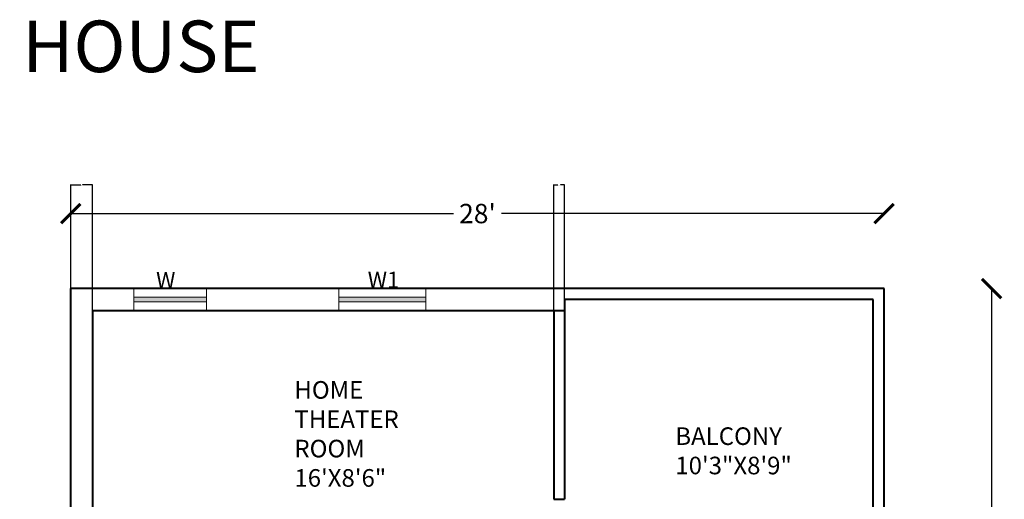
# Model space of a CAD drawing. Units: inches. Extents: x 182 to 1022, y -617 to 111.
# Tile 33 of 33: x 615 to 1022, y -87 to 111. Entities that reach past the tile are written whole.
import ezdxf

# ---------------------------------------------------------------- set-up
doc = ezdxf.new("R2010")
doc.units = ezdxf.units.IN
doc.header["$MEASUREMENT"] = 0
for name, color, linetype, lineweight in [('A-ANNO-DIMS', 2, 'Continuous', 18), ('A-ANNO-IDEN', 1, 'Continuous', 18), ('A-ANNO-TEXT', 8, 'Continuous', 20), ('A-AREA-IDEN', 8, 'Continuous', 18), ('A-GLAZ-PATT', 5, 'Continuous', 13), ('wall', 1, 'Continuous', 40), ('wind', 5, 'Continuous', 20)]:
    doc.layers.add(name, color=color, linetype=linetype, lineweight=lineweight)
doc.styles.get("Standard").update_dxf_attribs({"font": 'arial.ttf'})
doc.dimstyles.get("Standard").update_dxf_attribs({"dimtxt": 0.18, "dimasz": 0.18, "dimexe": 0.18, "dimexo": 0.0625, "dimgap": 0.09, "dimtad": 0, "dimtih": 1, "dimtoh": 1, "dimdec": 1, "dimzin": 0, "dimdsep": 46, "dimlunit": 4, "dimtxsty": 'Standard', "dimcen": 0.09, "dimadec": 0, "dimazin": 0, "dimtfac": 1, "dimtdec": 1, "dimtofl": 0, "dimtmove": 0, "dimatfit": 3, "dimfxl": 1, "dimtolj": 1, "dimtzin": 0, "dimarcsym": 0})

# ---------------------------------------------------------------- blocks, each defined once
blk = doc.blocks.new('_ArchTick')
at = {"color": 0, "linetype": 'ByBlock', "const_width": 0.15}
blk.add_lwpolyline([(-0.5, -0.5), (0.5, 0.5)], dxfattribs=at)
blk = doc.blocks.new('*D7')
at = {"layer": 'A-ANNO-DIMS', "color": 0, "lineweight": -2, "transparency": 16777216}
for p, q in [((636.3, 30.62), (794.45, 30.62)), ((972.3, 30.62), (814.16, 30.62))]:
    blk.add_line(p, q, dxfattribs=at)
at = {"layer": 'Defpoints', "color": 0, "transparency": 16777216}
for p in [(972.3, 30.62), (636.3, -0.37), (972.3, -0.37)]:
    blk.add_point(p, dxfattribs=at)
at = {"layer": 'A-ANNO-DIMS', "color": 0, "lineweight": -2, "transparency": 16777216, "xscale": 8, "yscale": 8, "zscale": 8, "rotation": 180}
blk.add_blockref('_ArchTick', (636.3, 30.62), dxfattribs=at)
at = {"layer": 'A-ANNO-DIMS', "color": 0, "lineweight": -2, "transparency": 16777216, "xscale": 8, "yscale": 8, "zscale": 8}
blk.add_blockref('_ArchTick', (972.3, 30.62), dxfattribs=at)
at = {"layer": 'A-ANNO-DIMS', "color": 0, "transparency": 16777216, "insert": (804.3, 30.62), "char_height": 8, "attachment_point": 5}
blk.add_mtext("\\A1;28'", dxfattribs=at)
blk = doc.blocks.new('*D8')
at = {"layer": 'A-ANNO-DIMS', "color": 0, "lineweight": -2, "transparency": 16777216}
for p, q in [((1016.69, -0.37), (1016.69, -260.42)), ((1016.69, -540.37), (1016.69, -280.32))]:
    blk.add_line(p, q, dxfattribs=at)
at = {"layer": 'Defpoints', "color": 0, "transparency": 16777216}
for p in [(972.3, -0.37), (972.3, -540.37), (1016.69, -540.37)]:
    blk.add_point(p, dxfattribs=at)
at = {"layer": 'A-ANNO-DIMS', "color": 0, "lineweight": -2, "transparency": 16777216, "xscale": 8, "yscale": 8, "zscale": 8}
for p, rotation in [((1016.69, -0.37), 90), ((1016.69, -540.37), 270)]:
    blk.add_blockref('_ArchTick', p, dxfattribs=dict(at, rotation=rotation))
at = {"layer": 'A-ANNO-DIMS', "color": 0, "transparency": 16777216, "insert": (1016.69, -270.37), "char_height": 8, "attachment_point": 5, "rotation": 90}
blk.add_mtext("\\A1;45'", dxfattribs=at)
blk = doc.blocks.new('*D41')
at = {"layer": 'A-ANNO-DIMS', "color": 0, "lineweight": -2, "transparency": 16777216}
for p, q in [((636.3, -0.31), (636.3, 42.61)), ((636.48, 42.43), (640.48, 42.43)), ((645.12, 42.43), (641.13, 42.43)), ((645.3, -9.31), (645.3, 42.61))]:
    blk.add_line(p, q, dxfattribs=at)
at = {"layer": 'A-ANNO-DIMS', "color": 0, "transparency": 16777216}
for points in [[(636.48, 42.46), (636.48, 42.4), (636.3, 42.43)], [(645.12, 42.46), (645.12, 42.4), (645.3, 42.43)]]:
    blk.add_solid(points, dxfattribs=at)
at = {"layer": 'Defpoints', "color": 0, "transparency": 16777216}
for p in [(645.3, 42.43), (636.3, -0.37), (645.3, -9.37)]:
    blk.add_point(p, dxfattribs=at)
at = {"layer": 'A-ANNO-DIMS', "color": 0, "transparency": 16777216, "insert": (640.8, 42.43), "char_height": 0.18, "attachment_point": 5}
blk.add_mtext('\\A1;0\'-9"', dxfattribs=at)
blk = doc.blocks.new('*D42')
at = {"layer": 'A-ANNO-DIMS', "color": 0, "lineweight": -2, "transparency": 16777216}
for p, q in [((835.8, -9.31), (835.8, 42.61)), ((835.98, 42.43), (837.52, 42.43)), ((840.12, 42.43), (838.59, 42.43)), ((840.3, -4.81), (840.3, 42.61))]:
    blk.add_line(p, q, dxfattribs=at)
at = {"layer": 'A-ANNO-DIMS', "color": 0, "transparency": 16777216}
for points in [[(835.98, 42.46), (835.98, 42.4), (835.8, 42.43)], [(840.12, 42.46), (840.12, 42.4), (840.3, 42.43)]]:
    blk.add_solid(points, dxfattribs=at)
at = {"layer": 'Defpoints', "color": 0, "transparency": 16777216}
for p in [(840.3, 42.43), (840.3, -4.87), (835.8, -9.37)]:
    blk.add_point(p, dxfattribs=at)
at = {"layer": 'A-ANNO-DIMS', "color": 0, "transparency": 16777216, "insert": (838.05, 42.43), "char_height": 0.18, "attachment_point": 5}
blk.add_mtext('\\A1;0\'-4 1/2"', dxfattribs=at)

msp = doc.modelspace()

# ---------------------------------------------------------------- hatches: boundary and pattern name
at = {"layer": 'A-GLAZ-PATT'}
h = msp.add_hatch(color=256, dxfattribs=at)
h.dxf.hatch_style = 1
h.paths.add_polyline_path([(692.35, -3.87), (662.35, -3.87), (662.35, -5.87), (692.35, -5.87)])
h.paths.add_polyline_path([(783.03, -3.87), (747.03, -3.87), (747.03, -5.87), (783.03, -5.87)])
h.paths.add_polyline_path([(641.8, -252.37), (639.8, -252.37), (639.8, -288.37), (641.8, -288.37)])
h.paths.add_polyline_path([(968.8, -258.37), (966.8, -258.37), (966.8, -282.37), (968.8, -282.37)])
h.paths.add_polyline_path([(968.8, -132.92), (966.8, -132.92), (966.8, -168.92), (968.8, -168.92)])
h.paths.add_polyline_path([(940.3, -534.87), (904.3, -534.87), (904.3, -536.87), (940.3, -536.87)])

# ---------------------------------------------------------------- linework, layer by layer
at = {"layer": 'wall'}
for p, q in [((636.3, -540.37), (636.3, -0.37)), ((972.3, -0.37), (636.3, -0.37)), ((972.3, -540.37), (972.3, -0.37)), ((840.3, -4.87), (840.3, -87.37)), ((967.8, -4.87), (840.3, -4.87)), ((967.8, -117.37), (967.8, -4.87)), ((645.3, -9.37), (645.3, -540.37)), ((645.3, -9.37), (840.3, -9.37)), ((835.8, -9.37), (835.8, -87.37)), ((835.8, -87.37), (840.3, -87.37))]:
    msp.add_line(p, q, dxfattribs=at)
at = {"layer": 'wind'}
for p, q in [((662.35, -9.37), (662.35, -0.37)), ((662.35, -3.87), (692.35, -3.87)), ((692.35, -9.37), (692.35, -0.37)), ((747.03, -9.37), (747.03, -0.37)), ((747.03, -3.87), (783.03, -3.87)), ((783.03, -9.37), (783.03, -0.37)), ((662.35, -5.87), (692.35, -5.87)), ((747.03, -5.87), (783.03, -5.87))]:
    msp.add_line(p, q, dxfattribs=at)

# ---------------------------------------------------------------- texts
at = {"layer": 'A-ANNO-IDEN'}
for s, height, p in [('W', 6.65, (671.54, -0.18)), ('W1', 6.652, (758.97, -0.07))]:
    msp.add_text(s, height=height, dxfattribs=at).set_placement(p)
at = {"layer": 'A-ANNO-TEXT', "insert": (424.27, 110.32), "char_height": 21.2807, "attachment_point": 1}
msp.add_mtext_dynamic_manual_height_columns('WEST FACING HOUSE', width=345.7385, gutter_width=3.55, heights=[0], dxfattribs=at)
at = {"layer": 'A-AREA-IDEN', "char_height": 7.2703, "attachment_point": 1}
for s, width, insert in [('HOME THEATER ROOM        16\'X8\'6"', 48.6806, (728.67, -38.59)), ('    BALCONY\\P    10\'3"X8\'9"', 65.8887, (877.15, -57.7))]:
    msp.add_mtext_dynamic_manual_height_columns(s, width=width, gutter_width=1.21, heights=[0], dxfattribs=dict(at, insert=insert))

# ---------------------------------------------------------------- dimensions: what is measured, and where the dimension line sits
at = {"layer": 'A-ANNO-DIMS'}
for base, p1, p2, override, picture, middle in [((645.3, 42.43), (636.3, -0.37), (645.3, -9.37), {"dimdec": 1, "dimlfac": 1, "dimrnd": 0, "dimzin": 1, "dimdsep": 46, "dimlunit": 4, "dimfrac": 2}, '*D41', (640.8, 42.43)), ((840.3, 42.43), (835.8, -9.37), (840.3, -4.87), {"dimdec": 1, "dimlfac": 1, "dimrnd": 0, "dimzin": 1, "dimdsep": 46, "dimlunit": 4, "dimfrac": 2}, '*D42', (838.05, 42.43)), ((972.3, 30.62), (636.3, -0.37), (972.3, -0.37), {"dimtxt": 8, "dimasz": 8, "dimgap": 3, "dimblk1": 'ArchTick', "dimblk2": 'ArchTick', "dimsah": 1, "dimse1": 1, "dimse2": 1, "dimclrd": 0, "dimclre": 0, "dimclrt": 0}, '*D7', (804.3, 30.62))]:
    dim = msp.add_linear_dim(base=base, p1=p1, p2=p2, dimstyle='Standard', override=override, dxfattribs=at)
    dim.commit()
    dim.dimension.update_dxf_attribs({"geometry": picture, "text_midpoint": middle})
dim = msp.add_linear_dim(base=(1016.69, -540.37), p1=(972.3, -0.37), p2=(972.3, -540.37), angle=90, dimstyle='Standard', override={"dimtxt": 8, "dimasz": 8, "dimgap": 3, "dimtih": 0, "dimblk1": 'ArchTick', "dimblk2": 'ArchTick', "dimsah": 1, "dimse1": 1, "dimse2": 1, "dimclrd": 0, "dimclre": 0, "dimclrt": 0}, dxfattribs=at)
dim.commit()
dim.dimension.update_dxf_attribs({"geometry": '*D8', "text_midpoint": (1016.69, -270.37)})

doc.saveas('drawing.dxf')
